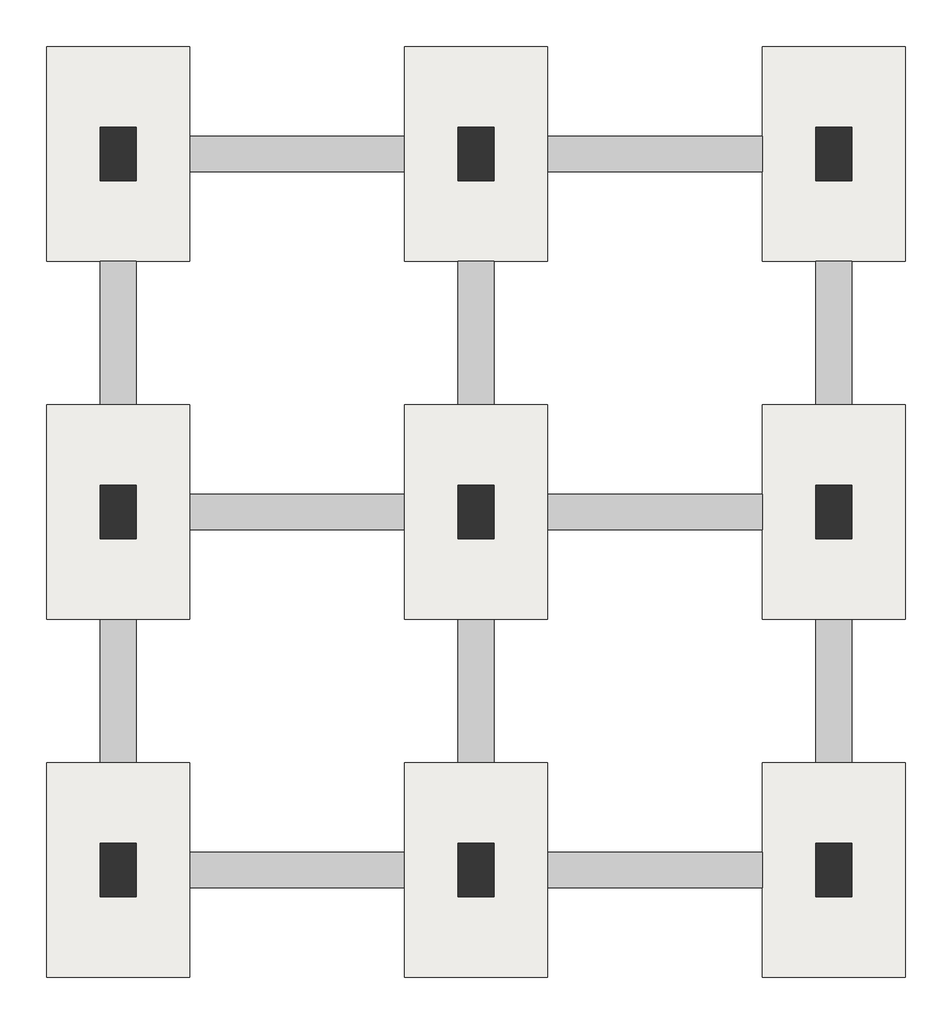
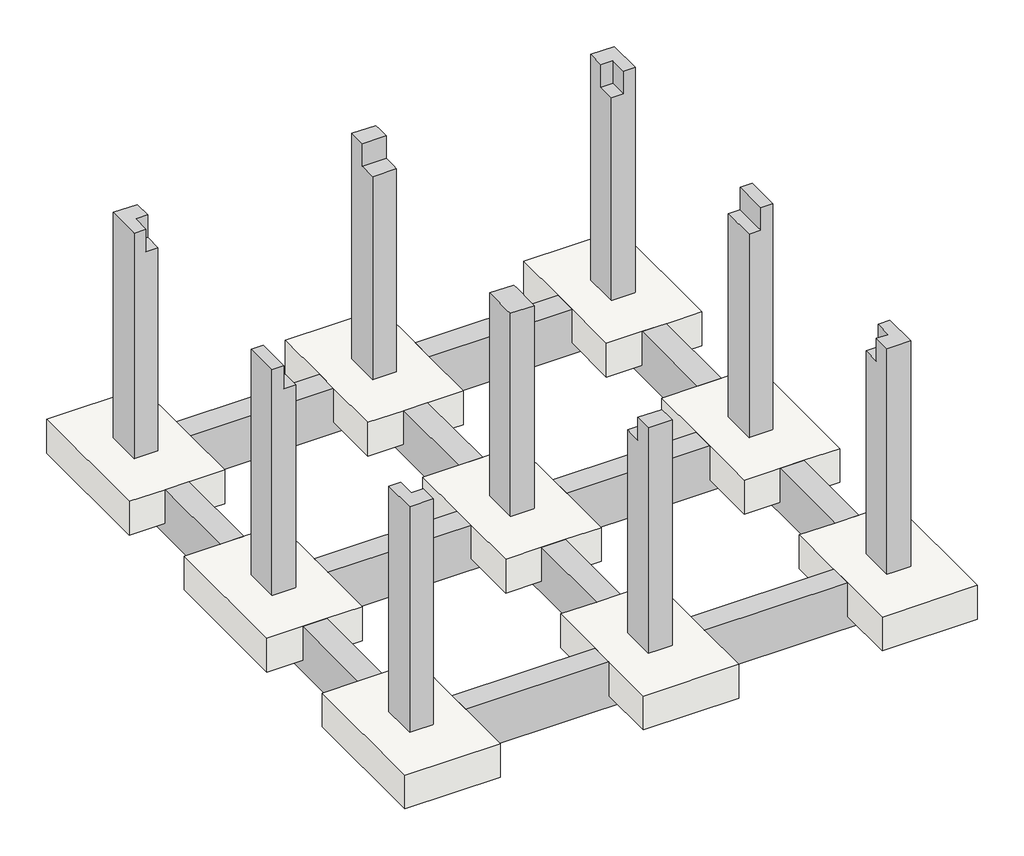
# One storey: 9 columns, 9 slabs, 6 beams.
"""IFC4 building model written with IfcOpenShell, lengths in millimetres."""

from ifc_helpers import new_model, si_unit, frame, origin, place, context, project, spatial, polyline, outline, extrude, faceted_brep, element, save

model = new_model("IFC4")

# Units and contexts
model_context = context("Model", 3, world=origin())
ifc_project = project(units=[si_unit("LENGTHUNIT", "METRE", prefix="MILLI")], contexts=[model_context])

# Site, building, storey
site = spatial("IfcSite", under=ifc_project)
building = spatial("IfcBuilding", under=site)
storey = spatial("IfcBuildingStorey", under=building, Elevation=0.0)

# Beams
placement = place(None, origin())
element("IfcBeam", 1, ObjectType="Concrete-Rectangular Beam : 300 x 600mm", at=placement, inside=storey, context=model_context, shape_type="Brep", body=[
    faceted_brep([(2518.7595868, 526.3372902, 0.0), (2518.7595868, 226.3372902, 0.0), (4318.7595868, 226.3372902, 0.0), (4318.7595868, 526.3372902, 0.0), (-481.2404132, 226.3372902, -450.0), (-931.2404132, 226.3372902, -450.0), (-1231.2404132, 226.3372902, -450.0), (-1231.2404132, 226.3372902, -600.0), (-931.2404132, 226.3372902, -600.0), (1768.7595868, 226.3372902, -600.0), (2068.7595868, 226.3372902, -600.0), (4768.7595868, 226.3372902, -600.0), (5068.7595868, 226.3372902, -600.0), (5068.7595868, 226.3372902, -450.0), (4768.7595868, 226.3372902, -450.0), (4318.7595868, 226.3372902, -450.0), (2518.7595868, 226.3372902, -450.0), (2068.7595868, 226.3372902, -450.0), (1768.7595868, 226.3372902, -450.0), (1318.7595868, 226.3372902, -450.0), (1318.7595868, 226.3372902, 0.0), (-481.2404132, 226.3372902, 0.0), (5068.7595868, 526.3372902, -600.0), (-1231.2404132, 526.3372902, -600.0), (-1231.2404132, 526.3372902, -450.0), (-481.2404132, 526.3372902, -450.0), (-481.2404132, 526.3372902, 0.0), (1318.7595868, 526.3372902, 0.0), (1318.7595868, 526.3372902, -450.0), (2518.7595868, 526.3372902, -450.0), (4318.7595868, 526.3372902, -450.0), (5068.7595868, 526.3372902, -450.0)], [[[0, 1, 2, 3]], [[4, 5, 6, 7, 8, 9, 10, 11, 12, 13, 14, 15, 2, 1, 16, 17, 18, 19, 20, 21]], [[22, 12, 11, 10, 9, 8, 7, 23]], [[24, 25, 26, 27, 28, 29, 0, 3, 30, 31, 22, 23]], [[4, 25, 24, 6, 5]], [[25, 4, 21, 26]], [[16, 29, 28, 19, 18, 17]], [[29, 16, 1, 0]], [[19, 28, 27, 20]], [[26, 21, 20, 27]], [[30, 15, 14, 13, 31]], [[15, 30, 3, 2]], [[12, 22, 31, 13]], [[23, 7, 6, 24]]]),
])
element("IfcBeam", 2, ObjectType="Concrete-Rectangular Beam : 300 x 600mm", at=placement, inside=storey, context=model_context, shape_type="Brep", body=[
    faceted_brep([(4768.7595868, -1723.6627098, 0.0), (5068.7595868, -1723.6627098, 0.0), (5068.7595868, -523.6627098, 0.0), (4768.7595868, -523.6627098, 0.0), (5068.7595868, -4723.6627098, -450.0), (5068.7595868, -5773.6627098, -450.0), (5068.7595868, -5773.6627098, -600.0), (5068.7595868, 226.3372902, -600.0), (5068.7595868, 226.3372902, -450.0), (5068.7595868, -523.6627098, -450.0), (5068.7595868, -1723.6627098, -450.0), (5068.7595868, -3523.6627098, -450.0), (5068.7595868, -3523.6627098, 0.0), (5068.7595868, -4723.6627098, 0.0), (4768.7595868, 226.3372902, -600.0), (4768.7595868, -5773.6627098, -600.0), (4768.7595868, -5473.6627098, -600.0), (4768.7595868, -2773.6627098, -600.0), (4768.7595868, -2473.6627098, -600.0), (4768.7595868, -5773.6627098, -450.0), (4768.7595868, -5473.6627098, -450.0), (4768.7595868, -4723.6627098, -450.0), (4768.7595868, -4723.6627098, 0.0), (4768.7595868, -3523.6627098, 0.0), (4768.7595868, -3523.6627098, -450.0), (4768.7595868, -2773.6627098, -450.0), (4768.7595868, -2473.6627098, -450.0), (4768.7595868, -1723.6627098, -450.0), (4768.7595868, -523.6627098, -450.0), (4768.7595868, 226.3372902, -450.0)], [[[0, 1, 2, 3]], [[4, 5, 6, 7, 8, 9, 2, 1, 10, 11, 12, 13]], [[14, 7, 6, 15, 16, 17, 18]], [[19, 20, 21, 22, 23, 24, 25, 26, 27, 0, 3, 28, 29, 14, 18, 17, 16, 15]], [[7, 14, 29, 8]], [[4, 21, 20, 19, 5]], [[21, 4, 13, 22]], [[24, 11, 10, 27, 26, 25]], [[11, 24, 23, 12]], [[27, 10, 1, 0]], [[22, 13, 12, 23]], [[28, 9, 8, 29]], [[9, 28, 3, 2]], [[15, 6, 5, 19]]]),
])
element("IfcBeam", 3, ObjectType="Concrete-Rectangular Beam : 300 x 600mm", at=placement, inside=storey, context=model_context, shape_type="Brep", body=[
    faceted_brep([(2518.7595868, -5473.6627098, 0.0), (2518.7595868, -5773.6627098, 0.0), (4318.7595868, -5773.6627098, 0.0), (4318.7595868, -5473.6627098, 0.0), (-481.2404132, -5773.6627098, -450.0), (-1231.2404132, -5773.6627098, -450.0), (-1231.2404132, -5773.6627098, -600.0), (4768.7595868, -5773.6627098, -600.0), (4768.7595868, -5773.6627098, -450.0), (4318.7595868, -5773.6627098, -450.0), (2518.7595868, -5773.6627098, -450.0), (1318.7595868, -5773.6627098, -450.0), (1318.7595868, -5773.6627098, 0.0), (-481.2404132, -5773.6627098, 0.0), (4768.7595868, -5473.6627098, -600.0), (-1231.2404132, -5473.6627098, -600.0), (-931.2404132, -5473.6627098, -600.0), (1768.7595868, -5473.6627098, -600.0), (2068.7595868, -5473.6627098, -600.0), (-1231.2404132, -5473.6627098, -450.0), (-931.2404132, -5473.6627098, -450.0), (-481.2404132, -5473.6627098, -450.0), (-481.2404132, -5473.6627098, 0.0), (1318.7595868, -5473.6627098, 0.0), (1318.7595868, -5473.6627098, -450.0), (1768.7595868, -5473.6627098, -450.0), (2068.7595868, -5473.6627098, -450.0), (2518.7595868, -5473.6627098, -450.0), (4318.7595868, -5473.6627098, -450.0), (4768.7595868, -5473.6627098, -450.0)], [[[0, 1, 2, 3]], [[4, 5, 6, 7, 8, 9, 2, 1, 10, 11, 12, 13]], [[14, 7, 6, 15, 16, 17, 18]], [[19, 20, 21, 22, 23, 24, 25, 26, 27, 0, 3, 28, 29, 14, 18, 17, 16, 15]], [[7, 14, 29, 8]], [[4, 21, 20, 19, 5]], [[21, 4, 13, 22]], [[10, 27, 26, 25, 24, 11]], [[27, 10, 1, 0]], [[11, 24, 23, 12]], [[22, 13, 12, 23]], [[28, 9, 8, 29]], [[9, 28, 3, 2]], [[15, 6, 5, 19]]]),
])
element("IfcBeam", 4, ObjectType="Concrete-Rectangular Beam : 300 x 600mm", at=placement, inside=storey, context=model_context, shape_type="Brep", body=[
    faceted_brep([(-1231.2404132, -4723.6627098, 0.0), (-931.2404132, -4723.6627098, 0.0), (-931.2404132, -3523.6627098, 0.0), (-1231.2404132, -3523.6627098, 0.0), (-1231.2404132, 226.3372902, -600.0), (-1231.2404132, -5473.6627098, -600.0), (-1231.2404132, -5473.6627098, -450.0), (-1231.2404132, -4723.6627098, -450.0), (-1231.2404132, -3523.6627098, -450.0), (-1231.2404132, -1723.6627098, -450.0), (-1231.2404132, -1723.6627098, 0.0), (-1231.2404132, -523.6627098, 0.0), (-1231.2404132, -523.6627098, -450.0), (-1231.2404132, 226.3372902, -450.0), (-931.2404132, 226.3372902, -600.0), (-931.2404132, -2473.6627098, -600.0), (-931.2404132, -2773.6627098, -600.0), (-931.2404132, -5473.6627098, -600.0), (-931.2404132, 226.3372902, -450.0), (-931.2404132, -523.6627098, -450.0), (-931.2404132, -523.6627098, 0.0), (-931.2404132, -1723.6627098, 0.0), (-931.2404132, -1723.6627098, -450.0), (-931.2404132, -2473.6627098, -450.0), (-931.2404132, -2773.6627098, -450.0), (-931.2404132, -3523.6627098, -450.0), (-931.2404132, -4723.6627098, -450.0), (-931.2404132, -5473.6627098, -450.0)], [[[0, 1, 2, 3]], [[4, 5, 6, 7, 0, 3, 8, 9, 10, 11, 12, 13]], [[4, 14, 15, 16, 17, 5]], [[17, 16, 15, 14, 18, 19, 20, 21, 22, 23, 24, 25, 2, 1, 26, 27]], [[14, 4, 13, 18]], [[5, 17, 27, 6]], [[26, 7, 6, 27]], [[7, 26, 1, 0]], [[8, 25, 24, 23, 22, 9]], [[25, 8, 3, 2]], [[9, 22, 21, 10]], [[10, 21, 20, 11]], [[12, 19, 18, 13]], [[19, 12, 11, 20]]]),
])
element("IfcBeam", 5, ObjectType="Concrete-Rectangular Beam : 300 x 600mm", at=placement, inside=storey, context=model_context, shape_type="Brep", body=[
    faceted_brep([(1768.7595868, -4723.6627098, 0.0), (2068.7595868, -4723.6627098, 0.0), (2068.7595868, -3523.6627098, 0.0), (1768.7595868, -3523.6627098, 0.0), (1768.7595868, 226.3372902, -600.0), (1768.7595868, -2473.6627098, -600.0), (1768.7595868, -2773.6627098, -600.0), (1768.7595868, -5473.6627098, -600.0), (1768.7595868, -5473.6627098, -450.0), (1768.7595868, -4723.6627098, -450.0), (1768.7595868, -3523.6627098, -450.0), (1768.7595868, -2773.6627098, -450.0), (1768.7595868, -2473.6627098, -450.0), (1768.7595868, -1723.6627098, -450.0), (1768.7595868, -1723.6627098, 0.0), (1768.7595868, -523.6627098, 0.0), (1768.7595868, -523.6627098, -450.0), (1768.7595868, 226.3372902, -450.0), (2068.7595868, 226.3372902, -600.0), (2068.7595868, -2473.6627098, -600.0), (2068.7595868, -2773.6627098, -600.0), (2068.7595868, -5473.6627098, -600.0), (2068.7595868, 226.3372902, -450.0), (2068.7595868, -523.6627098, -450.0), (2068.7595868, -523.6627098, 0.0), (2068.7595868, -1723.6627098, 0.0), (2068.7595868, -1723.6627098, -450.0), (2068.7595868, -2473.6627098, -450.0), (2068.7595868, -2773.6627098, -450.0), (2068.7595868, -3523.6627098, -450.0), (2068.7595868, -4723.6627098, -450.0), (2068.7595868, -5473.6627098, -450.0)], [[[0, 1, 2, 3]], [[4, 5, 6, 7, 8, 9, 0, 3, 10, 11, 12, 13, 14, 15, 16, 17]], [[4, 18, 19, 20, 21, 7, 6, 5]], [[21, 20, 19, 18, 22, 23, 24, 25, 26, 27, 28, 29, 2, 1, 30, 31]], [[18, 4, 17, 22]], [[7, 21, 31, 8]], [[30, 9, 8, 31]], [[9, 30, 1, 0]], [[10, 29, 28, 27, 26, 13, 12, 11]], [[29, 10, 3, 2]], [[13, 26, 25, 14]], [[14, 25, 24, 15]], [[16, 23, 22, 17]], [[23, 16, 15, 24]]]),
])
element("IfcBeam", 6, ObjectType="Concrete-Rectangular Beam : 300 x 600mm", at=placement, inside=storey, context=model_context, shape_type="SweptSolid", body=[
    extrude(outline(polyline([(0.0, 2518.7595868), (-450.0, 2518.7595868), (-450.0, 2068.7595868), (-600.0, 2068.7595868), (-600.0, 4768.7595868), (-450.0, 4768.7595868), (-450.0, 4318.7595868), (0.0, 4318.7595868), (0.0, 2518.7595868)])), frame((0.0, -2773.6627098, 0.0), z_axis=(0.0, 1.0, 0.0), x_axis=(0.0, 0.0, 1.0)), (0.0, 0.0, 1.0), 300.0),
    extrude(outline(polyline([(-450.0, -931.2404132), (-600.0, -931.2404132), (-600.0, 1768.7595868), (-450.0, 1768.7595868), (-450.0, 1318.7595868), (0.0, 1318.7595868), (0.0, -481.2404132), (-450.0, -481.2404132), (-450.0, -931.2404132)])), frame((0.0, -2773.6627098, 0.0), z_axis=(0.0, 1.0, 0.0), x_axis=(0.0, 0.0, 1.0)), (0.0, 0.0, 1.0), 300.0),
])

# Columns
element("IfcColumn", 7, ObjectType="Concrete-Rectangular-Column : 300 x 450mm", at=placement, inside=storey, context=model_context, shape_type="Brep", body=[
    faceted_brep([(-1231.2404132, -5848.6627098, 3000.0), (-931.2404132, -5848.6627098, 3000.0), (-931.2404132, -5623.6627098, 3000.0), (-1081.2404132, -5623.6627098, 3000.0), (-1081.2404132, -5398.6627098, 3000.0), (-1231.2404132, -5398.6627098, 3000.0), (-1231.2404132, -5848.6627098, 0.0), (-1231.2404132, -5398.6627098, 0.0), (-931.2404132, -5398.6627098, 0.0), (-931.2404132, -5848.6627098, 0.0), (-931.2404132, -5398.6627098, 2700.0), (-931.2404132, -5623.6627098, 2700.0), (-1081.2404132, -5398.6627098, 2700.0), (-1081.2404132, -5623.6627098, 2700.0)], [[[0, 1, 2, 3, 4, 5]], [[6, 7, 8, 9]], [[1, 0, 6, 9]], [[9, 8, 10, 11, 2, 1]], [[8, 7, 5, 4, 12, 10]], [[0, 5, 7, 6]], [[12, 13, 11, 10]], [[13, 3, 2, 11]], [[3, 13, 12, 4]]]),
])
element("IfcColumn", 8, ObjectType="Concrete-Rectangular-Column : 300 x 450mm", at=placement, inside=storey, context=model_context, shape_type="Brep", body=[
    faceted_brep([(1768.7595868, -5848.6627098, 3000.0), (2068.7595868, -5848.6627098, 3000.0), (2068.7595868, -5773.6627098, 3000.0), (2068.7595868, -5623.6627098, 3000.0), (1768.7595868, -5623.6627098, 3000.0), (1768.7595868, -5773.6627098, 3000.0), (1768.7595868, -5848.6627098, 0.0), (1768.7595868, -5398.6627098, 0.0), (2068.7595868, -5398.6627098, 0.0), (2068.7595868, -5848.6627098, 0.0), (2068.7595868, -5398.6627098, 2700.0), (2068.7595868, -5473.6627098, 2700.0), (2068.7595868, -5623.6627098, 2700.0), (1768.7595868, -5398.6627098, 2700.0), (1768.7595868, -5623.6627098, 2700.0), (1768.7595868, -5473.6627098, 2700.0)], [[[0, 1, 2, 3, 4, 5]], [[6, 7, 8, 9]], [[1, 0, 6, 9]], [[9, 8, 10, 11, 12, 3, 2, 1]], [[8, 7, 13, 10]], [[7, 6, 0, 5, 4, 14, 15, 13]], [[14, 12, 11, 10, 13, 15]], [[12, 14, 4, 3]]]),
])
element("IfcColumn", 9, ObjectType="Concrete-Rectangular-Column : 300 x 450mm", at=placement, inside=storey, context=model_context, shape_type="Brep", body=[
    faceted_brep([(4768.7595868, -5848.6627098, 3000.0), (5068.7595868, -5848.6627098, 3000.0), (5068.7595868, -5398.6627098, 3000.0), (4918.7595868, -5398.6627098, 3000.0), (4918.7595868, -5623.6627098, 3000.0), (4768.7595868, -5623.6627098, 3000.0), (4768.7595868, -5848.6627098, 0.0), (4768.7595868, -5398.6627098, 0.0), (5068.7595868, -5398.6627098, 0.0), (5068.7595868, -5848.6627098, 0.0), (4768.7595868, -5398.6627098, 2700.0), (4918.7595868, -5398.6627098, 2700.0), (4768.7595868, -5623.6627098, 2700.0), (4918.7595868, -5623.6627098, 2700.0)], [[[0, 1, 2, 3, 4, 5]], [[6, 7, 8, 9]], [[1, 0, 6, 9]], [[2, 1, 9, 8]], [[8, 7, 10, 11, 3, 2]], [[7, 6, 0, 5, 12, 10]], [[12, 13, 11, 10]], [[13, 4, 3, 11]], [[4, 13, 12, 5]]]),
])
element("IfcColumn", 10, ObjectType="Concrete-Rectangular-Column : 300 x 450mm", at=placement, inside=storey, context=model_context, shape_type="Brep", body=[
    faceted_brep([(-1231.2404132, -2398.6627098, 3000.0), (-1231.2404132, -2848.6627098, 3000.0), (-1081.2404132, -2848.6627098, 3000.0), (-1081.2404132, -2398.6627098, 3000.0), (-1231.2404132, -2848.6627098, 0.0), (-1231.2404132, -2398.6627098, 0.0), (-931.2404132, -2398.6627098, 0.0), (-931.2404132, -2848.6627098, 0.0), (-931.2404132, -2848.6627098, 2400.0), (-931.2404132, -2848.6627098, 2700.0), (-1081.2404132, -2848.6627098, 2700.0), (-1231.2404132, -2848.6627098, 2400.0), (-931.2404132, -2398.6627098, 2400.0), (-931.2404132, -2398.6627098, 2700.0), (-1231.2404132, -2398.6627098, 2400.0), (-1081.2404132, -2398.6627098, 2700.0)], [[[0, 1, 2, 3]], [[4, 5, 6, 7]], [[4, 7, 8, 9, 10, 2, 1, 11]], [[7, 6, 12, 13, 9, 8]], [[6, 5, 14, 0, 3, 15, 13, 12]], [[1, 0, 14, 5, 4, 11]], [[15, 10, 9, 13]], [[10, 15, 3, 2]]]),
])
element("IfcColumn", 11, ObjectType="Concrete-Rectangular-Column : 300 x 450mm", at=placement, inside=storey, context=model_context, shape_type="Brep", body=[
    faceted_brep([(1768.7595868, -2848.6627098, 0.0), (1768.7595868, -2398.6627098, 0.0), (2068.7595868, -2398.6627098, 0.0), (2068.7595868, -2848.6627098, 0.0), (2068.7595868, -2848.6627098, 2400.0), (2068.7595868, -2848.6627098, 2700.0), (1768.7595868, -2848.6627098, 2700.0), (1768.7595868, -2848.6627098, 2400.0), (2068.7595868, -2398.6627098, 2400.0), (2068.7595868, -2398.6627098, 2700.0), (2068.7595868, -2473.6627098, 2700.0), (2068.7595868, -2773.6627098, 2700.0), (1768.7595868, -2398.6627098, 2400.0), (1768.7595868, -2398.6627098, 2700.0), (1768.7595868, -2773.6627098, 2700.0), (1768.7595868, -2473.6627098, 2700.0)], [[[0, 1, 2, 3]], [[0, 3, 4, 5, 6, 7]], [[3, 2, 8, 9, 10, 11, 5, 4]], [[2, 1, 12, 13, 9, 8]], [[1, 0, 7, 6, 14, 15, 13, 12]], [[6, 5, 11, 10, 9, 13, 15, 14]]]),
])
element("IfcColumn", 12, ObjectType="Concrete-Rectangular-Column : 300 x 450mm", at=placement, inside=storey, context=model_context, shape_type="Brep", body=[
    faceted_brep([(5068.7595868, -2848.6627098, 3000.0), (5068.7595868, -2398.6627098, 3000.0), (4918.7595868, -2398.6627098, 3000.0), (4918.7595868, -2848.6627098, 3000.0), (4768.7595868, -2848.6627098, 0.0), (4768.7595868, -2398.6627098, 0.0), (5068.7595868, -2398.6627098, 0.0), (5068.7595868, -2848.6627098, 0.0), (5068.7595868, -2848.6627098, 2400.0), (4918.7595868, -2848.6627098, 2700.0), (4768.7595868, -2848.6627098, 2700.0), (4768.7595868, -2848.6627098, 2400.0), (5068.7595868, -2398.6627098, 2400.0), (4768.7595868, -2398.6627098, 2400.0), (4768.7595868, -2398.6627098, 2700.0), (4918.7595868, -2398.6627098, 2700.0)], [[[0, 1, 2, 3]], [[4, 5, 6, 7]], [[4, 7, 8, 0, 3, 9, 10, 11]], [[1, 0, 8, 7, 6, 12]], [[6, 5, 13, 14, 15, 2, 1, 12]], [[5, 4, 11, 10, 14, 13]], [[9, 15, 14, 10]], [[15, 9, 3, 2]]]),
])
element("IfcColumn", 13, ObjectType="Concrete-Rectangular-Column : 300 x 450mm", at=placement, inside=storey, context=model_context, shape_type="Brep", body=[
    faceted_brep([(-931.2404132, 601.3372902, 3000.0), (-1231.2404132, 601.3372902, 3000.0), (-1231.2404132, 151.3372902, 3000.0), (-1081.2404132, 151.3372902, 3000.0), (-1081.2404132, 376.3372902, 3000.0), (-931.2404132, 376.3372902, 3000.0), (-1231.2404132, 151.3372902, 0.0), (-1231.2404132, 601.3372902, 0.0), (-931.2404132, 601.3372902, 0.0), (-931.2404132, 151.3372902, 0.0), (-931.2404132, 151.3372902, 2700.0), (-1081.2404132, 151.3372902, 2700.0), (-931.2404132, 376.3372902, 2700.0), (-1081.2404132, 376.3372902, 2700.0)], [[[0, 1, 2, 3, 4, 5]], [[6, 7, 8, 9]], [[6, 9, 10, 11, 3, 2]], [[9, 8, 0, 5, 12, 10]], [[1, 0, 8, 7]], [[2, 1, 7, 6]], [[12, 13, 11, 10]], [[13, 4, 3, 11]], [[4, 13, 12, 5]]]),
])
element("IfcColumn", 14, ObjectType="Concrete-Rectangular-Column : 300 x 450mm", at=placement, inside=storey, context=model_context, shape_type="Brep", body=[
    faceted_brep([(2068.7595868, 601.3372902, 3000.0), (1768.7595868, 601.3372902, 3000.0), (1768.7595868, 526.3372902, 3000.0), (1768.7595868, 376.3372902, 3000.0), (2068.7595868, 376.3372902, 3000.0), (2068.7595868, 526.3372902, 3000.0), (1768.7595868, 151.3372902, 0.0), (1768.7595868, 601.3372902, 0.0), (2068.7595868, 601.3372902, 0.0), (2068.7595868, 151.3372902, 0.0), (2068.7595868, 151.3372902, 2700.0), (1768.7595868, 151.3372902, 2700.0), (2068.7595868, 376.3372902, 2700.0), (2068.7595868, 226.3372902, 2700.0), (1768.7595868, 226.3372902, 2700.0), (1768.7595868, 376.3372902, 2700.0)], [[[0, 1, 2, 3, 4, 5]], [[6, 7, 8, 9]], [[6, 9, 10, 11]], [[9, 8, 0, 5, 4, 12, 13, 10]], [[1, 0, 8, 7]], [[7, 6, 11, 14, 15, 3, 2, 1]], [[12, 15, 14, 11, 10, 13]], [[15, 12, 4, 3]]]),
])
element("IfcColumn", 15, ObjectType="Concrete-Rectangular-Column : 300 x 450mm", at=placement, inside=storey, context=model_context, shape_type="Brep", body=[
    faceted_brep([(5068.7595868, 151.3372902, 3000.0), (5068.7595868, 601.3372902, 3000.0), (4768.7595868, 601.3372902, 3000.0), (4768.7595868, 376.3372902, 3000.0), (4918.7595868, 376.3372902, 3000.0), (4918.7595868, 151.3372902, 3000.0), (4768.7595868, 151.3372902, 0.0), (4768.7595868, 601.3372902, 0.0), (5068.7595868, 601.3372902, 0.0), (5068.7595868, 151.3372902, 0.0), (4918.7595868, 151.3372902, 2700.0), (4768.7595868, 151.3372902, 2700.0), (4768.7595868, 376.3372902, 2700.0), (4918.7595868, 376.3372902, 2700.0)], [[[0, 1, 2, 3, 4, 5]], [[6, 7, 8, 9]], [[6, 9, 0, 5, 10, 11]], [[1, 0, 9, 8]], [[2, 1, 8, 7]], [[7, 6, 11, 12, 3, 2]], [[13, 12, 11, 10]], [[4, 13, 10, 5]], [[13, 4, 3, 12]]]),
])

# Slabs
element("IfcSlab", 16, ObjectType="Footing-Rectangular : 1800 x 1200 x 450mm", at=placement, inside=storey, context=model_context, shape_type="Brep", body=[
    faceted_brep([(-1681.2404132, -6523.6627098, 0.0), (-481.2404132, -6523.6627098, 0.0), (-481.2404132, -5773.6627098, 0.0), (-481.2404132, -5473.6627098, 0.0), (-481.2404132, -4723.6627098, 0.0), (-931.2404132, -4723.6627098, 0.0), (-1231.2404132, -4723.6627098, 0.0), (-1681.2404132, -4723.6627098, 0.0), (-1681.2404132, -6523.6627098, -450.0), (-1681.2404132, -4723.6627098, -450.0), (-1231.2404132, -4723.6627098, -450.0), (-931.2404132, -4723.6627098, -450.0), (-481.2404132, -4723.6627098, -450.0), (-481.2404132, -5473.6627098, -450.0), (-481.2404132, -5773.6627098, -450.0), (-481.2404132, -6523.6627098, -450.0)], [[[0, 1, 2, 3, 4, 5, 6, 7]], [[8, 9, 10, 11, 12, 13, 14, 15]], [[1, 0, 8, 15]], [[4, 3, 2, 1, 15, 14, 13, 12]], [[7, 6, 5, 4, 12, 11, 10, 9]], [[0, 7, 9, 8]]]),
])
element("IfcSlab", 17, ObjectType="Footing-Rectangular : 1800 x 1200 x 450mm", at=placement, inside=storey, context=model_context, shape_type="Brep", body=[
    faceted_brep([(1318.7595868, -6523.6627098, 0.0), (2518.7595868, -6523.6627098, 0.0), (2518.7595868, -5773.6627098, 0.0), (2518.7595868, -5473.6627098, 0.0), (2518.7595868, -4723.6627098, 0.0), (2068.7595868, -4723.6627098, 0.0), (1768.7595868, -4723.6627098, 0.0), (1318.7595868, -4723.6627098, 0.0), (1318.7595868, -5473.6627098, 0.0), (1318.7595868, -5773.6627098, 0.0), (1318.7595868, -6523.6627098, -450.0), (1318.7595868, -5773.6627098, -450.0), (1318.7595868, -5473.6627098, -450.0), (1318.7595868, -4723.6627098, -450.0), (1768.7595868, -4723.6627098, -450.0), (2068.7595868, -4723.6627098, -450.0), (2518.7595868, -4723.6627098, -450.0), (2518.7595868, -5473.6627098, -450.0), (2518.7595868, -5773.6627098, -450.0), (2518.7595868, -6523.6627098, -450.0)], [[[0, 1, 2, 3, 4, 5, 6, 7, 8, 9]], [[10, 11, 12, 13, 14, 15, 16, 17, 18, 19]], [[1, 0, 10, 19]], [[4, 3, 2, 1, 19, 18, 17, 16]], [[7, 6, 5, 4, 16, 15, 14, 13]], [[0, 9, 8, 7, 13, 12, 11, 10]]]),
])
element("IfcSlab", 18, ObjectType="Footing-Rectangular : 1800 x 1200 x 450mm", at=placement, inside=storey, context=model_context, shape_type="Brep", body=[
    faceted_brep([(4318.7595868, -6523.6627098, 0.0), (5518.7595868, -6523.6627098, 0.0), (5518.7595868, -4723.6627098, 0.0), (5068.7595868, -4723.6627098, 0.0), (4768.7595868, -4723.6627098, 0.0), (4318.7595868, -4723.6627098, 0.0), (4318.7595868, -5473.6627098, 0.0), (4318.7595868, -5773.6627098, 0.0), (4318.7595868, -6523.6627098, -450.0), (4318.7595868, -5773.6627098, -450.0), (4318.7595868, -5473.6627098, -450.0), (4318.7595868, -4723.6627098, -450.0), (4768.7595868, -4723.6627098, -450.0), (5068.7595868, -4723.6627098, -450.0), (5518.7595868, -4723.6627098, -450.0), (5518.7595868, -6523.6627098, -450.0)], [[[0, 1, 2, 3, 4, 5, 6, 7]], [[8, 9, 10, 11, 12, 13, 14, 15]], [[1, 0, 8, 15]], [[2, 1, 15, 14]], [[5, 4, 3, 2, 14, 13, 12, 11]], [[0, 7, 6, 5, 11, 10, 9, 8]]]),
])
element("IfcSlab", 19, ObjectType="Footing-Rectangular : 1800 x 1200 x 450mm", at=placement, inside=storey, context=model_context, shape_type="Brep", body=[
    faceted_brep([(-1681.2404132, -3523.6627098, 0.0), (-1231.2404132, -3523.6627098, 0.0), (-931.2404132, -3523.6627098, 0.0), (-481.2404132, -3523.6627098, 0.0), (-481.2404132, -2773.6627098, 0.0), (-481.2404132, -2473.6627098, 0.0), (-481.2404132, -1723.6627098, 0.0), (-931.2404132, -1723.6627098, 0.0), (-1231.2404132, -1723.6627098, 0.0), (-1681.2404132, -1723.6627098, 0.0), (-1681.2404132, -3523.6627098, -450.0), (-1681.2404132, -1723.6627098, -450.0), (-1231.2404132, -1723.6627098, -450.0), (-931.2404132, -1723.6627098, -450.0), (-481.2404132, -1723.6627098, -450.0), (-481.2404132, -2473.6627098, -450.0), (-481.2404132, -2773.6627098, -450.0), (-481.2404132, -3523.6627098, -450.0), (-931.2404132, -3523.6627098, -450.0), (-1231.2404132, -3523.6627098, -450.0)], [[[0, 1, 2, 3, 4, 5, 6, 7, 8, 9]], [[10, 11, 12, 13, 14, 15, 16, 17, 18, 19]], [[3, 2, 1, 0, 10, 19, 18, 17]], [[6, 5, 4, 3, 17, 16, 15, 14]], [[9, 8, 7, 6, 14, 13, 12, 11]], [[0, 9, 11, 10]]]),
])
element("IfcSlab", 20, ObjectType="Footing-Rectangular : 1800 x 1200 x 450mm", at=placement, inside=storey, context=model_context, shape_type="Brep", body=[
    faceted_brep([(1318.7595868, -3523.6627098, 0.0), (1768.7595868, -3523.6627098, 0.0), (2068.7595868, -3523.6627098, 0.0), (2518.7595868, -3523.6627098, 0.0), (2518.7595868, -2773.6627098, 0.0), (2518.7595868, -2473.6627098, 0.0), (2518.7595868, -1723.6627098, 0.0), (2068.7595868, -1723.6627098, 0.0), (1768.7595868, -1723.6627098, 0.0), (1318.7595868, -1723.6627098, 0.0), (1318.7595868, -2473.6627098, 0.0), (1318.7595868, -2773.6627098, 0.0), (1318.7595868, -3523.6627098, -450.0), (1318.7595868, -2773.6627098, -450.0), (1318.7595868, -2473.6627098, -450.0), (1318.7595868, -1723.6627098, -450.0), (1768.7595868, -1723.6627098, -450.0), (2068.7595868, -1723.6627098, -450.0), (2518.7595868, -1723.6627098, -450.0), (2518.7595868, -2473.6627098, -450.0), (2518.7595868, -2773.6627098, -450.0), (2518.7595868, -3523.6627098, -450.0), (2068.7595868, -3523.6627098, -450.0), (1768.7595868, -3523.6627098, -450.0)], [[[0, 1, 2, 3, 4, 5, 6, 7, 8, 9, 10, 11]], [[12, 13, 14, 15, 16, 17, 18, 19, 20, 21, 22, 23]], [[3, 2, 1, 0, 12, 23, 22, 21]], [[6, 5, 4, 3, 21, 20, 19, 18]], [[9, 8, 7, 6, 18, 17, 16, 15]], [[0, 11, 10, 9, 15, 14, 13, 12]]]),
])
element("IfcSlab", 21, ObjectType="Footing-Rectangular : 1800 x 1200 x 450mm", at=placement, inside=storey, context=model_context, shape_type="Brep", body=[
    faceted_brep([(4318.7595868, -3523.6627098, 0.0), (4768.7595868, -3523.6627098, 0.0), (5068.7595868, -3523.6627098, 0.0), (5518.7595868, -3523.6627098, 0.0), (5518.7595868, -1723.6627098, 0.0), (5068.7595868, -1723.6627098, 0.0), (4768.7595868, -1723.6627098, 0.0), (4318.7595868, -1723.6627098, 0.0), (4318.7595868, -2473.6627098, 0.0), (4318.7595868, -2773.6627098, 0.0), (4318.7595868, -3523.6627098, -450.0), (4318.7595868, -2773.6627098, -450.0), (4318.7595868, -2473.6627098, -450.0), (4318.7595868, -1723.6627098, -450.0), (4768.7595868, -1723.6627098, -450.0), (5068.7595868, -1723.6627098, -450.0), (5518.7595868, -1723.6627098, -450.0), (5518.7595868, -3523.6627098, -450.0), (5068.7595868, -3523.6627098, -450.0), (4768.7595868, -3523.6627098, -450.0)], [[[0, 1, 2, 3, 4, 5, 6, 7, 8, 9]], [[10, 11, 12, 13, 14, 15, 16, 17, 18, 19]], [[3, 2, 1, 0, 10, 19, 18, 17]], [[4, 3, 17, 16]], [[7, 6, 5, 4, 16, 15, 14, 13]], [[0, 9, 8, 7, 13, 12, 11, 10]]]),
])
element("IfcSlab", 22, ObjectType="Footing-Rectangular : 1800 x 1200 x 450mm", at=placement, inside=storey, context=model_context, shape_type="Brep", body=[
    faceted_brep([(-1681.2404132, -523.6627098, 0.0), (-1231.2404132, -523.6627098, 0.0), (-931.2404132, -523.6627098, 0.0), (-481.2404132, -523.6627098, 0.0), (-481.2404132, 226.3372902, 0.0), (-481.2404132, 526.3372902, 0.0), (-481.2404132, 1276.3372902, 0.0), (-1681.2404132, 1276.3372902, 0.0), (-1681.2404132, -523.6627098, -450.0), (-1681.2404132, 1276.3372902, -450.0), (-481.2404132, 1276.3372902, -450.0), (-481.2404132, 526.3372902, -450.0), (-481.2404132, 226.3372902, -450.0), (-481.2404132, -523.6627098, -450.0), (-931.2404132, -523.6627098, -450.0), (-1231.2404132, -523.6627098, -450.0)], [[[0, 1, 2, 3, 4, 5, 6, 7]], [[8, 9, 10, 11, 12, 13, 14, 15]], [[3, 2, 1, 0, 8, 15, 14, 13]], [[6, 5, 4, 3, 13, 12, 11, 10]], [[7, 6, 10, 9]], [[0, 7, 9, 8]]]),
])
element("IfcSlab", 23, ObjectType="Footing-Rectangular : 1800 x 1200 x 450mm", at=placement, inside=storey, context=model_context, shape_type="Brep", body=[
    faceted_brep([(1318.7595868, -523.6627098, 0.0), (1768.7595868, -523.6627098, 0.0), (2068.7595868, -523.6627098, 0.0), (2518.7595868, -523.6627098, 0.0), (2518.7595868, 226.3372902, 0.0), (2518.7595868, 526.3372902, 0.0), (2518.7595868, 1276.3372902, 0.0), (1318.7595868, 1276.3372902, 0.0), (1318.7595868, 526.3372902, 0.0), (1318.7595868, 226.3372902, 0.0), (1318.7595868, -523.6627098, -450.0), (1318.7595868, 226.3372902, -450.0), (1318.7595868, 526.3372902, -450.0), (1318.7595868, 1276.3372902, -450.0), (2518.7595868, 1276.3372902, -450.0), (2518.7595868, 526.3372902, -450.0), (2518.7595868, 226.3372902, -450.0), (2518.7595868, -523.6627098, -450.0), (2068.7595868, -523.6627098, -450.0), (1768.7595868, -523.6627098, -450.0)], [[[0, 1, 2, 3, 4, 5, 6, 7, 8, 9]], [[10, 11, 12, 13, 14, 15, 16, 17, 18, 19]], [[3, 2, 1, 0, 10, 19, 18, 17]], [[6, 5, 4, 3, 17, 16, 15, 14]], [[7, 6, 14, 13]], [[0, 9, 8, 7, 13, 12, 11, 10]]]),
])
element("IfcSlab", 24, ObjectType="Footing-Rectangular : 1800 x 1200 x 450mm", at=placement, inside=storey, context=model_context, shape_type="Brep", body=[
    faceted_brep([(4318.7595868, -523.6627098, 0.0), (4768.7595868, -523.6627098, 0.0), (5068.7595868, -523.6627098, 0.0), (5518.7595868, -523.6627098, 0.0), (5518.7595868, 1276.3372902, 0.0), (4318.7595868, 1276.3372902, 0.0), (4318.7595868, 526.3372902, 0.0), (4318.7595868, 226.3372902, 0.0), (4318.7595868, -523.6627098, -450.0), (4318.7595868, 226.3372902, -450.0), (4318.7595868, 526.3372902, -450.0), (4318.7595868, 1276.3372902, -450.0), (5518.7595868, 1276.3372902, -450.0), (5518.7595868, -523.6627098, -450.0), (5068.7595868, -523.6627098, -450.0), (4768.7595868, -523.6627098, -450.0)], [[[0, 1, 2, 3, 4, 5, 6, 7]], [[8, 9, 10, 11, 12, 13, 14, 15]], [[3, 2, 1, 0, 8, 15, 14, 13]], [[4, 3, 13, 12]], [[5, 4, 12, 11]], [[0, 7, 6, 5, 11, 10, 9, 8]]]),
])

save(model, "model.ifc")

# Revit data of these elements
# Grids (mm)
#   "1": line (-8645.912, -5623.663) -> (22277.801, -5623.663)
#   "2": line (-8645.912, -2623.663) -> (22277.801, -2623.663)
#   "3": line (-8645.912, 376.337) -> (22277.801, 376.337)
#   "4": line (-1081.24, 5432.396) -> (-1081.24, -9031.921)
#   "5": line (1918.76, 5432.396) -> (1918.76, -9031.921)
#   "6": line (4918.76, 5432.396) -> (4918.76, -9031.921)
# Type "Concrete-Rectangular Beam : 300 x 600mm"
#   Length [instance default] = 1.524 m
#   b = 0.3 m
#   h = 0.6 m
#   Structural Material [instance default] = Concrete, Cast-in-Place gray
#   Assembly Code = ""
# Type "Concrete-Rectangular-Column : 300 x 450mm"
#   b = 0.3 m
#   h = 0.45 m
#   Structural Material [instance default] = Concrete, Cast-in-Place gray
# Type "Footing-Rectangular : 1800 x 1200 x 450mm"
#   Width = 1.2 m
#   Length = 1.8 m
#   Foundation Thickness = 0.45 m
#   Structural Material [instance default] = Concrete - Cast-in-Place Concrete
#   Assembly Code = ""
# Elements 1, 2, 3, 4, 5, 6 (IfcBeam, "Concrete-Rectangular Beam : 300 x 600mm")
#   Structural Material = Concrete, Cast-in-Place gray
#   Phase Created = New Construction
#   Materials on its faces: "Concrete, Cast-in-Place gray"
# Elements 7, 8, 9, 10, 11, 12, 13, 14, 15 (IfcColumn, "Concrete-Rectangular-Column : 300 x 450mm")
#   Structural Material = Concrete, Cast-in-Place gray
#   Phase Created = New Construction
#   Materials on its faces: "Concrete, Cast-in-Place gray"
# Elements 16, 17, 18, 19, 20, 21, 22, 23, 24 (IfcSlab, "Footing-Rectangular : 1800 x 1200 x 450mm")
#   Structural Material = Concrete - Cast-in-Place Concrete
#   Phase Created = New Construction
#   Materials on its faces: "Concrete - Cast-in-Place Concrete"
# Materials
#   "Concrete, Cast-in-Place gray": class "Concrete", colour RGB 192 192 192, transparency 0, Description = "Cast-in-place concrete", Cost = 0
#   "Concrete - Cast-in-Place Concrete": class "Concrete", colour RGB 192 192 192, transparency 0, Cost = 0
